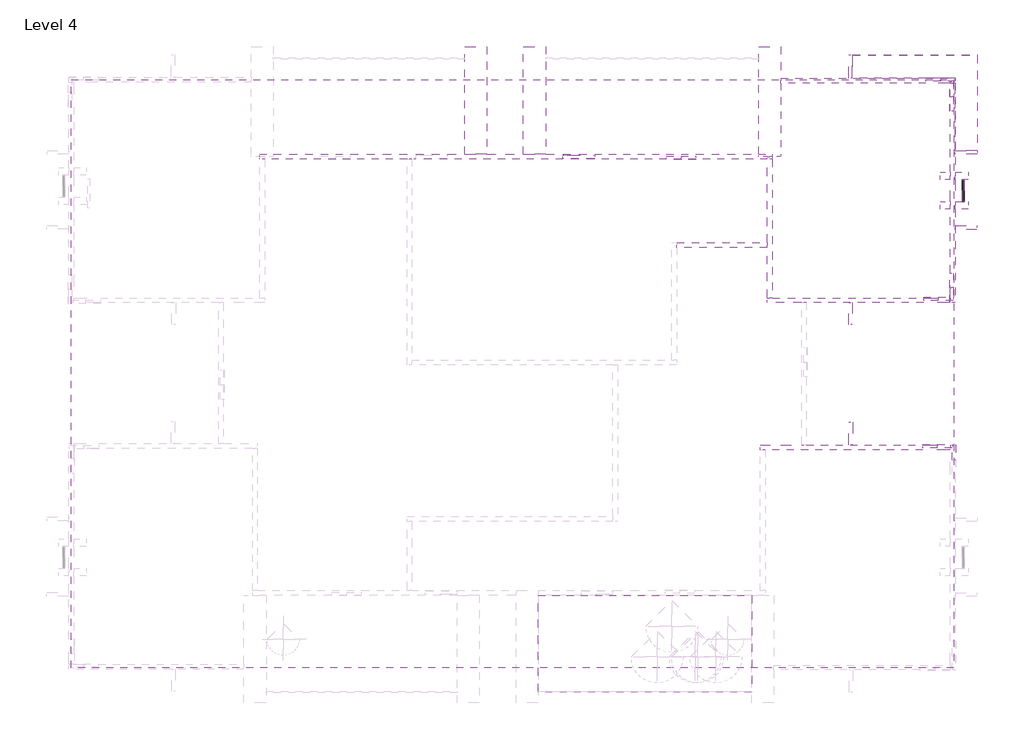
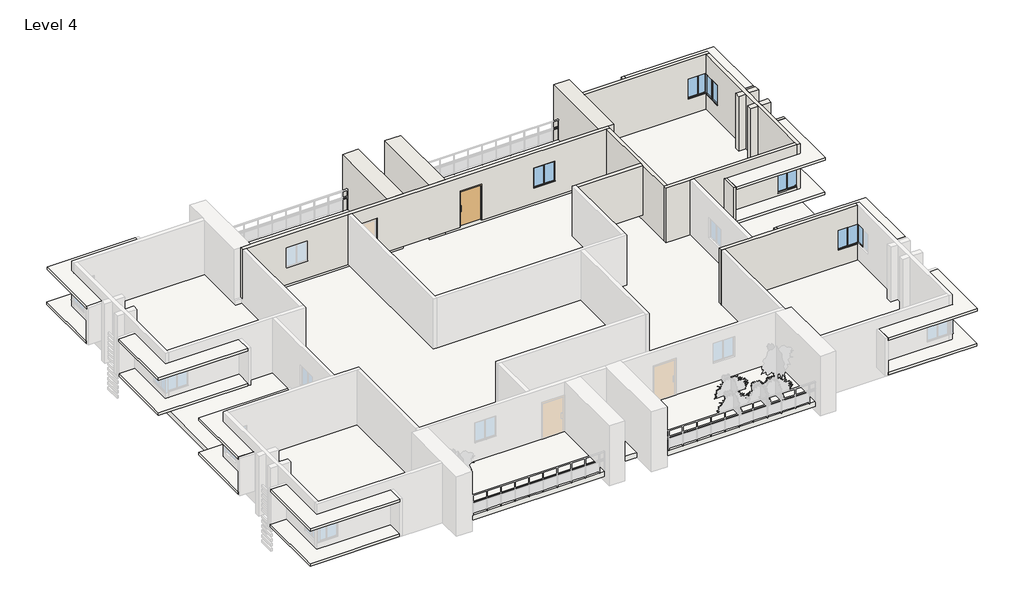
# One storey, part 3 of 4: 31 walls, 13 windows, 4 slabs, 1 door.
"""IFC4 building model written with IfcOpenShell, lengths in millimetres."""

from ifc_helpers import new_model, si_unit, frame, origin, place, context, project, spatial, polyline, outline, extrude, faceted_brep, transform, mapped, element, save
from components import door_15d3c954, window_20ff4747

model = new_model("IFC4")

# Units and contexts
model_context = context("Model", 3, world=origin())
ifc_project = project(units=[si_unit("LENGTHUNIT", "METRE", prefix="MILLI")], contexts=[model_context])

# Site, building, storey
site = spatial("IfcSite", under=ifc_project)
building = spatial("IfcBuilding", under=site)
storey = spatial("IfcBuildingStorey", under=building, Name="Level 4", Elevation=9144.0)

# Door
placement = place(None, origin())
door_shape = door_15d3c954(model_context)
element("IfcDoor", 1, ObjectType="Door-Passage-Single-Flush-Dbl_Acting : 48\" x 96\"", at=placement, inside=storey, context=model_context, shape_type="MappedRepresentation", body=[
    mapped(door_shape, transform((6249.0520665, 12804.5205944, 10972.8), x_axis=(1.0, 0.0, 0.0), y_axis=(0.0, 1.0, 0.0), z_axis=(0.0, 0.0, 1.0))),
])

# Slabs
element("IfcSlab", 2, ObjectType="Generic - 2'", at=placement, inside=storey, context=model_context, shape_type="SweptSolid", body=[
    extrude(outline(polyline([(21793.8520665, 16006.5548886), (21793.8520665, -8377.4451114), (-14782.1479335, -8377.4451114), (-14782.1479335, 16006.5548886), (21793.8520665, 16006.5548886)])), frame((0.0, 0.0, 10363.2), z_axis=(0.0, 0.0, 1.0), x_axis=(1.0, 0.0, 0.0)), (0.0, 0.0, 1.0), 304.8),
])
element("IfcSlab", 3, ObjectType="Generic - 2' gray", at=placement, inside=storey, context=model_context, shape_type="SweptSolid", body=[
    extrude(outline(polyline([(13411.8520665, -5363.830811), (13411.8520665, -9380.382663), (4572.6520665, -9380.382663), (4572.6520665, -5363.830811), (13411.8520665, -5363.830811)])), frame((0.0, 0.0, 10668.0), z_axis=(0.0, 0.0, 1.0), x_axis=(1.0, 0.0, 0.0)), (0.0, 0.0, 1.0), 304.8),
    extrude(outline(polyline([(-6704.9479335, -5363.1461695), (1219.8520665, -5363.1461695), (1219.8520665, -9380.382663), (-6704.9479335, -9380.382663), (-6704.9479335, -5363.1461695)])), frame((0.0, 0.0, 10668.0), z_axis=(0.0, 0.0, 1.0), x_axis=(1.0, 0.0, 0.0)), (0.0, 0.0, 1.0), 304.8),
    extrude(outline(polyline([(13716.6520665, 12912.4705944), (4877.4520665, 12912.4705944), (4877.4520665, 16886.1559451), (13716.6520665, 16886.1559451), (13716.6520665, 12912.4705944)])), frame((0.0, 0.0, 10668.0), z_axis=(0.0, 0.0, 1.0), x_axis=(1.0, 0.0, 0.0)), (0.0, 0.0, 1.0), 304.8),
    extrude(outline(polyline([(-6400.1479335, 12912.4705944), (-6400.1479335, 16886.1559451), (1524.6520665, 16886.1559451), (1524.6520665, 12912.4705944), (-6400.1479335, 12912.4705944)])), frame((0.0, 0.0, 10668.0), z_axis=(0.0, 0.0, 1.0), x_axis=(1.0, 0.0, 0.0)), (0.0, 0.0, 1.0), 304.8),
])
element("IfcSlab", 4, ObjectType="Generic - 6\"", at=placement, inside=storey, context=model_context, shape_type="SweptSolid", body=[
    extrude(outline(polyline([(-10616.5479335, -9354.6604699), (-15798.1479335, -9354.6604699), (-15798.1479335, -5392.2604699), (-14883.7479335, -5392.2604699), (-14883.7479335, -8338.6604699), (-14883.7479335, -8440.2604699), (-10616.5479335, -8440.2604699), (-10616.5479335, -9354.6604699)])), frame((0.0, 0.0, 11125.2), z_axis=(0.0, 0.0, 1.0), x_axis=(1.0, 0.0, 0.0)), (0.0, 0.0, 1.0), 152.4),
    extrude(outline(polyline([(-10633.1034654, 1834.0395301), (-10633.1034654, 919.6395301), (-14883.7479335, 919.6395301), (-14883.7479335, -2128.3604699), (-15775.8097154, -2128.3604699), (-15775.8097154, 1834.0395301), (-10633.1034654, 1834.0395301)])), frame((0.0, 0.0, 11125.2), z_axis=(0.0, 0.0, 1.0), x_axis=(1.0, 0.0, 0.0)), (0.0, 0.0, 1.0), 152.4),
    extrude(outline(polyline([(-10616.5479335, 5846.5548886), (-15798.1479335, 5846.5548886), (-15798.1479335, 9808.9548886), (-14883.7479335, 9808.9548886), (-14883.7479335, 6862.5548886), (-14883.7479335, 6760.9548886), (-10616.5479335, 6760.9548886), (-10616.5479335, 5846.5548886)])), frame((0.0, 0.0, 11125.2), z_axis=(0.0, 0.0, 1.0), x_axis=(1.0, 0.0, 0.0)), (0.0, 0.0, 1.0), 152.4),
    extrude(outline(polyline([(-10633.1034654, 17035.2548886), (-10633.1034654, 16120.8548886), (-14883.7479335, 16120.8548886), (-14883.7479335, 13072.8548886), (-15775.8097154, 13072.8548886), (-15775.8097154, 17035.2548886), (-10633.1034654, 17035.2548886)])), frame((0.0, 0.0, 11125.2), z_axis=(0.0, 0.0, 1.0), x_axis=(1.0, 0.0, 0.0)), (0.0, 0.0, 1.0), 152.4),
    extrude(outline(polyline([(17590.1520665, 17035.2548886), (22771.7520665, 17035.2548886), (22771.7520665, 13072.8548886), (21857.3520665, 13072.8548886), (21857.3520665, 16019.2548886), (21857.3520665, 16070.0548886), (17590.1520665, 16070.0548886), (17590.1520665, 16120.8548886), (17590.1520665, 17035.2548886)])), frame((0.0, 0.0, 11125.2), z_axis=(0.0, 0.0, 1.0), x_axis=(1.0, 0.0, 0.0)), (0.0, 0.0, 1.0), 152.4),
    extrude(outline(polyline([(17606.7075984, 5846.5548886), (17606.7075984, 6760.9548886), (21857.3520665, 6760.9548886), (21857.3520665, 9808.9548886), (22749.4138484, 9808.9548886), (22749.4138484, 5846.5548886), (17606.7075984, 5846.5548886)])), frame((0.0, 0.0, 11125.2), z_axis=(0.0, 0.0, 1.0), x_axis=(1.0, 0.0, 0.0)), (0.0, 0.0, 1.0), 152.4),
    extrude(outline(polyline([(17590.1520665, 1807.9548886), (22771.7520665, 1807.9548886), (22771.7520665, -2154.4451114), (21857.3520665, -2154.4451114), (21857.3520665, 791.9548886), (21857.3520665, 893.5548886), (17590.1520665, 893.5548886), (17590.1520665, 1807.9548886)])), frame((0.0, 0.0, 11125.2), z_axis=(0.0, 0.0, 1.0), x_axis=(1.0, 0.0, 0.0)), (0.0, 0.0, 1.0), 152.4),
    extrude(outline(polyline([(17606.7075984, -9380.7451114), (17606.7075984, -8466.3451114), (21857.3520665, -8466.3451114), (21857.3520665, -5418.3451114), (22749.4138484, -5418.3451114), (22749.4138484, -9380.7451114), (17606.7075984, -9380.7451114)])), frame((0.0, 0.0, 11125.2), z_axis=(0.0, 0.0, 1.0), x_axis=(1.0, 0.0, 0.0)), (0.0, 0.0, 1.0), 152.4),
])
element("IfcSlab", 5, ObjectType="Generic - 6\"", at=placement, inside=storey, context=model_context, shape_type="SweptSolid", body=[
    extrude(outline(polyline([(-10617.0810044, -9363.7552779), (-15798.6810044, -9363.7552779), (-15798.6810044, -5401.3552779), (-14884.2810044, -5401.3552779), (-14884.2810044, -8347.7552779), (-14884.2810044, -8449.3552779), (-10617.0810044, -8449.3552779), (-10617.0810044, -9363.7552779)])), frame((0.0, 0.0, 13258.8), z_axis=(0.0, 0.0, 1.0), x_axis=(1.0, 0.0, 0.0)), (0.0, 0.0, 1.0), 152.4),
    extrude(outline(polyline([(-10633.6365363, 1824.9447221), (-10633.6365363, 910.5447221), (-14884.2810044, 910.5447221), (-14884.2810044, -2137.4552779), (-15776.3427863, -2137.4552779), (-15776.3427863, 1824.9447221), (-10633.6365363, 1824.9447221)])), frame((0.0, 0.0, 13258.8), z_axis=(0.0, 0.0, 1.0), x_axis=(1.0, 0.0, 0.0)), (0.0, 0.0, 1.0), 152.4),
    extrude(outline(polyline([(-10617.0810044, 5837.4600805), (-15798.6810044, 5837.4600805), (-15798.6810044, 9799.8600805), (-14884.2810044, 9799.8600805), (-14884.2810044, 6853.4600805), (-14884.2810044, 6751.8600805), (-10617.0810044, 6751.8600805), (-10617.0810044, 5837.4600805)])), frame((0.0, 0.0, 13258.8), z_axis=(0.0, 0.0, 1.0), x_axis=(1.0, 0.0, 0.0)), (0.0, 0.0, 1.0), 152.4),
    extrude(outline(polyline([(-10633.6365363, 17026.1600805), (-10633.6365363, 16111.7600805), (-14884.2810044, 16111.7600805), (-14884.2810044, 13063.7600805), (-15776.3427863, 13063.7600805), (-15776.3427863, 17026.1600805), (-10633.6365363, 17026.1600805)])), frame((0.0, 0.0, 13258.8), z_axis=(0.0, 0.0, 1.0), x_axis=(1.0, 0.0, 0.0)), (0.0, 0.0, 1.0), 152.4),
    extrude(outline(polyline([(17589.6189956, 17026.1600805), (22771.2189956, 17026.1600805), (22771.2189956, 13063.7600805), (21856.8189956, 13063.7600805), (21856.8189956, 16010.1600805), (21856.8189956, 16060.9600805), (17589.6189956, 16060.9600805), (17589.6189956, 16111.7600805), (17589.6189956, 17026.1600805)])), frame((0.0, 0.0, 13258.8), z_axis=(0.0, 0.0, 1.0), x_axis=(1.0, 0.0, 0.0)), (0.0, 0.0, 1.0), 152.4),
    extrude(outline(polyline([(17606.1745274, 5837.4600805), (17606.1745274, 6751.8600805), (21856.8189956, 6751.8600805), (21856.8189956, 9799.8600805), (22748.8807774, 9799.8600805), (22748.8807774, 5837.4600805), (17606.1745274, 5837.4600805)])), frame((0.0, 0.0, 13258.8), z_axis=(0.0, 0.0, 1.0), x_axis=(1.0, 0.0, 0.0)), (0.0, 0.0, 1.0), 152.4),
    extrude(outline(polyline([(17589.6189956, 1798.8600805), (22771.2189956, 1798.8600805), (22771.2189956, -2163.5399195), (21856.8189956, -2163.5399195), (21856.8189956, 782.8600805), (21856.8189956, 884.4600805), (17589.6189956, 884.4600805), (17589.6189956, 1798.8600805)])), frame((0.0, 0.0, 13258.8), z_axis=(0.0, 0.0, 1.0), x_axis=(1.0, 0.0, 0.0)), (0.0, 0.0, 1.0), 152.4),
    extrude(outline(polyline([(17606.1745274, -9389.8399195), (17606.1745274, -8475.4399195), (21856.8189956, -8475.4399195), (21856.8189956, -5427.4399195), (22748.8807774, -5427.4399195), (22748.8807774, -9389.8399195), (17606.1745274, -9389.8399195)])), frame((0.0, 0.0, 13258.8), z_axis=(0.0, 0.0, 1.0), x_axis=(1.0, 0.0, 0.0)), (0.0, 0.0, 1.0), 152.4),
])

# Walls
element("IfcWall", 6, ObjectType="Generic - 1'", at=placement, inside=storey, context=model_context, shape_type="SweptSolid", body=[
    extrude(outline(polyline([(22386.1027846, 11871.0705944), (21857.3520665, 11871.0705944), (21857.3520665, 12175.8705944), (22386.1027846, 12175.8705944), (22386.1027846, 11871.0705944)])), frame((0.0, 0.0, 10363.2), z_axis=(0.0, 0.0, 1.0), x_axis=(1.0, 0.0, 0.0)), (0.0, 0.0, 1.0), 3657.6),
])
element("IfcWall", 7, ObjectType="Generic - 1'", at=placement, inside=storey, context=model_context, shape_type="SweptSolid", body=[
    extrude(outline(polyline([(21235.7605971, 12175.8705944), (21654.1520665, 12175.8705944), (21654.1520665, 11871.0705944), (21235.7605971, 11871.0705944), (21235.7605971, 12175.8705944)])), frame((0.0, 0.0, 10363.2), z_axis=(0.0, 0.0, 1.0), x_axis=(1.0, 0.0, 0.0)), (0.0, 0.0, 1.0), 3657.6),
])
element("IfcWall", 8, ObjectType="Generic - 1'", at=placement, inside=storey, context=model_context, shape_type="SweptSolid", body=[
    extrude(outline(polyline([(22386.1027846, 10651.8705944), (21857.3520665, 10651.8705944), (21857.3520665, 10956.6705944), (22386.1027846, 10956.6705944), (22386.1027846, 10651.8705944)])), frame((0.0, 0.0, 10363.2), z_axis=(0.0, 0.0, 1.0), x_axis=(1.0, 0.0, 0.0)), (0.0, 0.0, 1.0), 3657.6),
])
element("IfcWall", 9, ObjectType="Generic - 1'", at=placement, inside=storey, context=model_context, shape_type="SweptSolid", body=[
    extrude(outline(polyline([(21235.7605971, 10956.6705944), (21654.1520665, 10956.6705944), (21654.1520665, 10651.8705944), (21235.7605971, 10651.8705944), (21235.7605971, 10956.6705944)])), frame((0.0, 0.0, 10363.2), z_axis=(0.0, 0.0, 1.0), x_axis=(1.0, 0.0, 0.0)), (0.0, 0.0, 1.0), 3657.6),
])
element("IfcWall", 10, ObjectType="Generic - 3'", at=placement, inside=storey, context=model_context, shape_type="SweptSolid", body=[
    extrude(outline(polyline([(2439.0520665, 17382.8705944), (2439.0520665, 12912.4705944), (1524.6520665, 12912.4705944), (1524.6520665, 17382.8705944), (2439.0520665, 17382.8705944)])), frame((0.0, 0.0, 10363.2), z_axis=(0.0, 0.0, 1.0), x_axis=(1.0, 0.0, 0.0)), (0.0, 0.0, 1.0), 3657.6),
])
element("IfcWall", 11, ObjectType="Generic - 3'", at=placement, inside=storey, context=model_context, shape_type="SweptSolid", body=[
    extrude(outline(polyline([(4877.4520665, 17382.8705944), (4877.4520665, 12912.4705944), (3963.0520665, 12912.4705944), (3963.0520665, 17382.8705944), (4877.4520665, 17382.8705944)])), frame((0.0, 0.0, 10363.2), z_axis=(0.0, 0.0, 1.0), x_axis=(1.0, 0.0, 0.0)), (0.0, 0.0, 1.0), 3657.6),
])
element("IfcWall", 12, ObjectType="Generic - 3'", at=placement, inside=storey, context=model_context, shape_type="Brep", body=[
    faceted_brep([(14631.0520665, 12810.8705944, 10363.2), (14631.0520665, 15866.8548886, 10363.2), (14631.0520665, 16070.0548886, 10363.2), (14631.0520665, 17382.8705944, 10363.2), (14631.0520665, 17382.8705944, 14020.8), (14631.0520665, 16070.0548886, 14020.8), (14631.0520665, 15866.8548886, 14020.8), (14631.0520665, 12912.4705944, 14020.8), (14631.0520665, 12912.4705944, 10972.8), (14631.0520665, 12810.8705944, 10972.8), (13716.6520665, 12810.8705944, 10363.2), (13716.6520665, 12810.8705944, 10972.8), (13716.6520665, 12912.4705944, 10972.8), (13716.6520665, 12912.4705944, 14020.8), (13716.6520665, 17382.8705944, 14020.8), (13716.6520665, 17382.8705944, 10363.2), (14275.4520665, 12810.8705944, 10363.2), (14072.2520665, 12810.8705944, 10363.2), (14275.4520665, 12912.4705944, 14020.8), (14275.4520665, 12810.8705944, 10972.8), (14072.2520665, 12810.8705944, 10972.8), (14275.4520665, 12912.4705944, 10972.8)], [[[0, 1, 2, 3, 4, 5, 6, 7, 8, 9]], [[10, 11, 12, 13, 14, 15]], [[3, 2, 1, 0, 16, 17, 10, 15]], [[4, 3, 15, 14]], [[7, 6, 5, 4, 14, 13, 18]], [[0, 9, 19, 20, 11, 10, 17, 16]], [[8, 21, 12, 11, 20, 19, 9]], [[8, 7, 18, 13, 12, 21]]]),
])
element("IfcWall", 13, ObjectType="Generic - 5\"", at=placement, inside=storey, context=model_context, shape_type="SweptSolid", body=[
    extrude(outline(polyline([(22145.9857703, 10956.6705944), (22145.9857703, 11871.0705944), (22222.1857703, 11871.0705944), (22222.1857703, 10956.6705944), (22145.9857703, 10956.6705944)])), frame((0.0, 0.0, 8712.2), z_axis=(0.0, 0.0, 1.0), x_axis=(1.0, 0.0, 0.0)), (0.0, 0.0, 1.0), 152.8735856),
])
element("IfcWall", 14, ObjectType="Generic - 5\"", at=placement, inside=storey, context=model_context, shape_type="SweptSolid", body=[
    extrude(outline(polyline([(22145.9857703, 10956.6705944), (22145.9857703, 11871.0705944), (22222.1857703, 11871.0705944), (22222.1857703, 10956.6705944), (22145.9857703, 10956.6705944)])), frame((0.0, 0.0, 9017.0), z_axis=(0.0, 0.0, 1.0), x_axis=(1.0, 0.0, 0.0)), (0.0, 0.0, 1.0), 152.8735856),
])
element("IfcWall", 15, ObjectType="Generic - 5\"", at=placement, inside=storey, context=model_context, shape_type="SweptSolid", body=[
    extrude(outline(polyline([(22145.9857703, 10956.6705944), (22145.9857703, 11871.0705944), (22222.1857703, 11871.0705944), (22222.1857703, 10956.6705944), (22145.9857703, 10956.6705944)])), frame((0.0, 0.0, 9296.4), z_axis=(0.0, 0.0, 1.0), x_axis=(1.0, 0.0, 0.0)), (0.0, 0.0, 1.0), 152.8735856),
])
element("IfcWall", 16, ObjectType="Generic - 5\"", at=placement, inside=storey, context=model_context, shape_type="SweptSolid", body=[
    extrude(outline(polyline([(22145.9857703, 10956.6705944), (22145.9857703, 11871.0705944), (22222.1857703, 11871.0705944), (22222.1857703, 10956.6705944), (22145.9857703, 10956.6705944)])), frame((0.0, 0.0, 9601.2), z_axis=(0.0, 0.0, 1.0), x_axis=(1.0, 0.0, 0.0)), (0.0, 0.0, 1.0), 152.8735856),
])
element("IfcWall", 17, ObjectType="Generic - 5\"", at=placement, inside=storey, context=model_context, shape_type="SweptSolid", body=[
    extrude(outline(polyline([(22145.9857703, 10956.6705944), (22145.9857703, 11871.0705944), (22222.1857703, 11871.0705944), (22222.1857703, 10956.6705944), (22145.9857703, 10956.6705944)])), frame((0.0, 0.0, 9906.0), z_axis=(0.0, 0.0, 1.0), x_axis=(1.0, 0.0, 0.0)), (0.0, 0.0, 1.0), 152.8735856),
])
element("IfcWall", 18, ObjectType="Generic - 5\"", at=placement, inside=storey, context=model_context, shape_type="SweptSolid", body=[
    extrude(outline(polyline([(22145.9857703, 10956.6705944), (22145.9857703, 11871.0705944), (22222.1857703, 11871.0705944), (22222.1857703, 10956.6705944), (22145.9857703, 10956.6705944)])), frame((0.0, 0.0, 10210.8), z_axis=(0.0, 0.0, 1.0), x_axis=(1.0, 0.0, 0.0)), (0.0, 0.0, 1.0), 152.8735856),
])
element("IfcWall", 19, ObjectType="Generic - 5\"", at=placement, inside=storey, context=model_context, shape_type="SweptSolid", body=[
    extrude(outline(polyline([(22145.9857703, 10956.6705944), (22145.9857703, 11871.0705944), (22222.1857703, 11871.0705944), (22222.1857703, 10956.6705944), (22145.9857703, 10956.6705944)])), frame((0.0, 0.0, 10617.2), z_axis=(0.0, 0.0, 1.0), x_axis=(1.0, 0.0, 0.0)), (0.0, 0.0, 1.0), 152.8735856),
])
element("IfcWall", 20, ObjectType="Generic - 5\"", at=placement, inside=storey, context=model_context, shape_type="SweptSolid", body=[
    extrude(outline(polyline([(22145.9857703, 10956.6705944), (22145.9857703, 11871.0705944), (22222.1857703, 11871.0705944), (22222.1857703, 10956.6705944), (22145.9857703, 10956.6705944)])), frame((0.0, 0.0, 10896.6), z_axis=(0.0, 0.0, 1.0), x_axis=(1.0, 0.0, 0.0)), (0.0, 0.0, 1.0), 152.8735856),
])
element("IfcWall", 21, ObjectType="Generic - 5\"", at=placement, inside=storey, context=model_context, shape_type="SweptSolid", body=[
    extrude(outline(polyline([(22145.9857703, 10956.6705944), (22145.9857703, 11871.0705944), (22222.1857703, 11871.0705944), (22222.1857703, 10956.6705944), (22145.9857703, 10956.6705944)])), frame((0.0, 0.0, 11176.0), z_axis=(0.0, 0.0, 1.0), x_axis=(1.0, 0.0, 0.0)), (0.0, 0.0, 1.0), 152.8735856),
])
element("IfcWall", 22, ObjectType="Generic - 5\"", at=placement, inside=storey, context=model_context, shape_type="SweptSolid", body=[
    extrude(outline(polyline([(22145.9857703, 10956.6705944), (22145.9857703, 11871.0705944), (22222.1857703, 11871.0705944), (22222.1857703, 10956.6705944), (22145.9857703, 10956.6705944)])), frame((0.0, 0.0, 11480.8), z_axis=(0.0, 0.0, 1.0), x_axis=(1.0, 0.0, 0.0)), (0.0, 0.0, 1.0), 152.8735856),
])
element("IfcWall", 23, ObjectType="Generic - 5\"", at=placement, inside=storey, context=model_context, shape_type="SweptSolid", body=[
    extrude(outline(polyline([(22145.9857703, 10956.6705944), (22145.9857703, 11871.0705944), (22222.1857703, 11871.0705944), (22222.1857703, 10956.6705944), (22145.9857703, 10956.6705944)])), frame((0.0, 0.0, 11785.6), z_axis=(0.0, 0.0, 1.0), x_axis=(1.0, 0.0, 0.0)), (0.0, 0.0, 1.0), 152.8735856),
])
element("IfcWall", 24, ObjectType="Generic - 5\"", at=placement, inside=storey, context=model_context, shape_type="SweptSolid", body=[
    extrude(outline(polyline([(22145.9857703, 10956.6705944), (22145.9857703, 11871.0705944), (22222.1857703, 11871.0705944), (22222.1857703, 10956.6705944), (22145.9857703, 10956.6705944)])), frame((0.0, 0.0, 12065.0), z_axis=(0.0, 0.0, 1.0), x_axis=(1.0, 0.0, 0.0)), (0.0, 0.0, 1.0), 152.8735856),
])
element("IfcWall", 25, ObjectType="Generic - 6\"", at=placement, inside=storey, context=model_context, shape_type="SweptSolid", body=[
    extrude(outline(polyline([(22771.7520665, 12914.1048886), (21857.3520665, 12914.1048886), (21857.3520665, 13066.5048886), (22771.7520665, 13066.5048886), (22771.7520665, 12914.1048886)])), frame((0.0, 0.0, 11125.2), z_axis=(0.0, 0.0, 1.0), x_axis=(1.0, 0.0, 0.0)), (0.0, 0.0, 1.0), 2286.0),
])
element("IfcWall", 26, ObjectType="Generic - 6\"", at=placement, inside=storey, context=model_context, shape_type="SweptSolid", body=[
    extrude(outline(polyline([(17590.1520665, 17035.2548886), (17590.1520665, 16070.0548886), (17437.7520665, 16070.0548886), (17437.7520665, 17035.2548886), (17590.1520665, 17035.2548886)])), frame((0.0, 0.0, 11125.2), z_axis=(0.0, 0.0, 1.0), x_axis=(1.0, 0.0, 0.0)), (0.0, 0.0, 1.0), 2286.0),
])
element("IfcWall", 27, ObjectType="Generic - 6\"", at=placement, inside=storey, context=model_context, shape_type="SweptSolid", body=[
    extrude(outline(polyline([(22748.8807774, 9799.8600805), (21857.3520665, 9799.8600805), (21857.3520665, 9952.2600805), (22748.8807774, 9952.2600805), (22748.8807774, 9799.8600805)])), frame((0.0, 0.0, 11125.2), z_axis=(0.0, 0.0, 1.0), x_axis=(1.0, 0.0, 0.0)), (0.0, 0.0, 1.0), 2286.0),
])
element("IfcWall", 28, ObjectType="Generic - 6\"", at=placement, inside=storey, context=model_context, shape_type="SweptSolid", body=[
    extrude(outline(polyline([(17441.6075984, 5850.1600805), (17441.6075984, 6760.9548886), (17594.0075984, 6760.9548886), (17594.0075984, 5850.1600805), (17441.6075984, 5850.1600805)])), frame((0.0, 0.0, 11125.2), z_axis=(0.0, 0.0, 1.0), x_axis=(1.0, 0.0, 0.0)), (0.0, 0.0, 1.0), 2286.0),
])
element("IfcWall", 29, ObjectType="Generic - 6\"", at=placement, inside=storey, context=model_context, shape_type="SweptSolid", body=[
    extrude(outline(polyline([(17595.9689956, 1807.9548886), (17595.9689956, 868.1548886), (17443.5689956, 868.1548886), (17443.5689956, 1807.9548886), (17595.9689956, 1807.9548886)])), frame((0.0, 0.0, 11125.2), z_axis=(0.0, 0.0, 1.0), x_axis=(1.0, 0.0, 0.0)), (0.0, 0.0, 1.0), 2286.0),
])
element("IfcWall", 30, ObjectType="Generic - 8\"", at=placement, inside=storey, context=model_context, shape_type="SweptSolid", body=[
    extrude(outline(polyline([(14072.2520665, 9051.6705944), (10313.0520665, 9051.6705944), (10313.0520665, 9254.8705944), (14072.2520665, 9254.8705944), (14072.2520665, 9051.6705944)])), frame((0.0, 0.0, 10972.8), z_axis=(0.0, 0.0, 1.0), x_axis=(1.0, 0.0, 0.0)), (0.0, 0.0, 1.0), 3048.0),
])
element("IfcWall", 31, ObjectType="Generic - 8\" gray", at=placement, inside=storey, context=model_context, shape_type="Brep", body=[
    faceted_brep([(21857.3520665, 16070.0548886, 10363.2), (14631.0520665, 16070.0548886, 10363.2), (14631.0520665, 16070.0548886, 14020.8), (21857.3520665, 16070.0548886, 14020.8), (20634.9770665, 16070.0548886, 11635.4804451), (21854.1770665, 16070.0548886, 11635.4804451), (21854.1770665, 16070.0548886, 12854.6804451), (20634.9770665, 16070.0548886, 12854.6804451), (14631.0520665, 15866.8548886, 10363.2), (21654.1520665, 15866.8548886, 10363.2), (21857.3520665, 15866.8548886, 10363.2), (21857.3520665, 15866.8548886, 11617.3280277), (21857.3520665, 15866.8548886, 12836.5280277), (21857.3520665, 15866.8548886, 14020.8), (21654.1520665, 15866.8548886, 14020.8), (14631.0520665, 15866.8548886, 14020.8), (20634.9770665, 15866.8548886, 12854.6804451), (21854.1770665, 15866.8548886, 12854.6804451), (21854.1770665, 15866.8548886, 11635.4804451), (20634.9770665, 15866.8548886, 11635.4804451)], [[[0, 1, 2, 3], [4, 5, 6, 7]], [[8, 9, 10, 11, 12, 13, 14, 15], [16, 17, 18, 19]], [[1, 0, 10, 9, 8]], [[3, 2, 15, 14, 13]], [[0, 3, 13, 12, 11, 10]], [[2, 1, 8, 15]], [[18, 17, 6, 5]], [[18, 5, 4, 19]], [[16, 7, 6, 17]], [[19, 4, 7, 16]]]),
])
element("IfcWall", 32, ObjectType="Generic - 8\" gray", at=placement, inside=storey, context=model_context, shape_type="Brep", body=[
    faceted_brep([(21857.3520665, 6760.9548886, 10363.2), (21857.3520665, 10651.8705944, 10363.2), (21857.3520665, 10956.6705944, 10363.2), (21857.3520665, 11871.0705944, 10363.2), (21857.3520665, 12175.8705944, 10363.2), (21857.3520665, 15866.8548886, 10363.2), (21857.3520665, 15866.8548886, 11617.3280277), (21857.3520665, 14696.4442594, 11617.3280277), (21857.3520665, 14696.4442594, 12836.5280277), (21857.3520665, 15866.8548886, 12836.5280277), (21857.3520665, 15866.8548886, 14020.8), (21857.3520665, 12175.8705944, 14020.8), (21857.3520665, 11871.0705944, 14020.8), (21857.3520665, 10956.6705944, 14020.8), (21857.3520665, 10651.8705944, 14020.8), (21857.3520665, 6760.9548886, 14020.8), (21857.3520665, 7997.1026284, 11470.2947232), (21857.3520665, 6777.9026284, 11470.2947232), (21857.3520665, 6777.9026284, 12689.4947232), (21857.3520665, 7997.1026284, 12689.4947232), (21654.1520665, 15866.8548886, 10363.2), (21654.1520665, 12175.8705944, 10363.2), (21654.1520665, 11871.0705944, 10363.2), (21654.1520665, 10956.6705944, 10363.2), (21654.1520665, 10651.8705944, 10363.2), (21654.1520665, 6964.1548886, 10363.2), (21654.1520665, 6760.9548886, 10363.2), (21654.1520665, 6760.9548886, 11421.1450479), (21654.1520665, 6760.9548886, 12640.3450479), (21654.1520665, 6760.9548886, 14020.8), (21654.1520665, 6964.1548886, 14020.8), (21654.1520665, 10651.8705944, 14020.8), (21654.1520665, 10956.6705944, 14020.8), (21654.1520665, 11871.0705944, 14020.8), (21654.1520665, 12175.8705944, 14020.8), (21654.1520665, 15866.8548886, 14020.8), (21654.1520665, 15866.8548886, 12836.5280277), (21654.1520665, 14696.4442594, 12836.5280277), (21654.1520665, 14696.4442594, 11617.3280277), (21654.1520665, 15866.8548886, 11617.3280277), (21654.1520665, 6777.9026284, 11470.2947232), (21654.1520665, 7997.1026284, 11470.2947232), (21654.1520665, 7997.1026284, 12689.4947232), (21654.1520665, 6777.9026284, 12689.4947232)], [[[0, 1, 2, 3, 4, 5, 6, 7, 8, 9, 10, 11, 12, 13, 14, 15], [16, 17, 18, 19]], [[20, 21, 22, 23, 24, 25, 26, 27, 28, 29, 30, 31, 32, 33, 34, 35, 36, 37, 38, 39], [40, 41, 42, 43]], [[5, 4, 3, 2, 1, 0, 26, 25, 24, 23, 22, 21, 20]], [[15, 14, 13, 12, 11, 10, 35, 34, 33, 32, 31, 30, 29]], [[0, 15, 29, 28, 27, 26]], [[5, 20, 39, 6]], [[35, 10, 9, 36]], [[38, 7, 6, 39]], [[8, 7, 38, 37]], [[8, 37, 36, 9]], [[16, 41, 40, 17]], [[18, 43, 42, 19]], [[19, 42, 41, 16]], [[43, 18, 17, 40]]]),
])
element("IfcWall", 33, ObjectType="Generic - 8\" gray", at=placement, inside=storey, context=model_context, shape_type="Brep", body=[
    faceted_brep([(14072.2520665, 6760.9548886, 10363.2), (15481.9520665, 6760.9548886, 10363.2), (15685.1520665, 6760.9548886, 10363.2), (21654.1520665, 6760.9548886, 10363.2), (21654.1520665, 6760.9548886, 11421.1450479), (20541.6213445, 6760.9548886, 11421.1450479), (20541.6213445, 6760.9548886, 12640.3450479), (21654.1520665, 6760.9548886, 12640.3450479), (21654.1520665, 6760.9548886, 14020.8), (15685.1520665, 6760.9548886, 14020.8), (15481.9520665, 6760.9548886, 14020.8), (14072.2520665, 6760.9548886, 14020.8), (21654.1520665, 6964.1548886, 10363.2), (14275.4520665, 6964.1548886, 10363.2), (14072.2520665, 6964.1548886, 10363.2), (14072.2520665, 6964.1548886, 14020.8), (14275.4520665, 6964.1548886, 14020.8), (21654.1520665, 6964.1548886, 14020.8), (21654.1520665, 6964.1548886, 12640.3450479), (20541.6213445, 6964.1548886, 12640.3450479), (20541.6213445, 6964.1548886, 11421.1450479), (21654.1520665, 6964.1548886, 11421.1450479)], [[[0, 1, 2, 3, 4, 5, 6, 7, 8, 9, 10, 11]], [[12, 13, 14, 15, 16, 17, 18, 19, 20, 21]], [[3, 2, 1, 0, 14, 13, 12]], [[11, 10, 9, 8, 17, 16, 15]], [[3, 12, 21, 4]], [[17, 8, 7, 18]], [[0, 11, 15, 14]], [[4, 21, 20, 5]], [[6, 5, 20, 19]], [[6, 19, 18, 7]]]),
])
element("IfcWall", 34, ObjectType="Generic - 8\" gray", at=placement, inside=storey, context=model_context, shape_type="Brep", body=[
    faceted_brep([(13767.4520665, 664.9548886, 10363.2), (13970.6520665, 664.9548886, 10363.2), (21654.1520665, 664.9548886, 10363.2), (21654.1520665, 664.9548886, 11635.4804451), (20505.783383, 664.9548886, 11635.4804451), (20505.783383, 664.9548886, 12854.6804451), (21654.1520665, 664.9548886, 12854.6804451), (21654.1520665, 664.9548886, 14020.8), (13970.6520665, 664.9548886, 14020.8), (13767.4520665, 664.9548886, 14020.8), (21654.1520665, 868.1548886, 10363.2), (15685.1520665, 868.1548886, 10363.2), (15481.9520665, 868.1548886, 10363.2), (13767.4520665, 868.1548886, 10363.2), (13767.4520665, 868.1548886, 14020.8), (15481.9520665, 868.1548886, 14020.8), (15685.1520665, 868.1548886, 14020.8), (21654.1520665, 868.1548886, 14020.8), (21654.1520665, 868.1548886, 12854.6804451), (20505.783383, 868.1548886, 12854.6804451), (20505.783383, 868.1548886, 11635.4804451), (21654.1520665, 868.1548886, 11635.4804451), (21654.1520665, 859.364485, 11635.4804451), (21654.1520665, 859.364485, 12854.6804451)], [[[0, 1, 2, 3, 4, 5, 6, 7, 8, 9]], [[10, 11, 12, 13, 14, 15, 16, 17, 18, 19, 20, 21]], [[2, 1, 0, 13, 12, 11, 10]], [[9, 8, 7, 17, 16, 15, 14]], [[2, 10, 21, 22, 3]], [[17, 7, 6, 23, 18]], [[0, 9, 14, 13]], [[3, 22, 21, 20, 4]], [[5, 4, 20, 19]], [[5, 19, 18, 23, 6]]]),
])
element("IfcWall", 35, ObjectType="Generic - 8\" gray", at=placement, inside=storey, context=model_context, shape_type="Brep", body=[
    faceted_brep([(-6958.9479335, 12912.4705944, 14020.8), (-6400.1479335, 12912.4705944, 14020.8), (1524.6520665, 12912.4705944, 14020.8), (2439.0520665, 12912.4705944, 14020.8), (3963.0520665, 12912.4705944, 14020.8), (4877.4520665, 12912.4705944, 14020.8), (13716.6520665, 12912.4705944, 14020.8), (14275.4520665, 12912.4705944, 14020.8), (14275.4520665, 12912.4705944, 10972.8), (13716.6520665, 12912.4705944, 10972.8), (6909.4520665, 12912.4705944, 10972.8), (6909.4520665, 12912.4705944, 13208.0), (5588.6520665, 12912.4705944, 13208.0), (5588.6520665, 12912.4705944, 10972.8), (813.4520665, 12912.4705944, 10972.8), (813.4520665, 12912.4705944, 13208.0), (-507.3479335, 12912.4705944, 13208.0), (-507.3479335, 12912.4705944, 10972.8), (-6400.1479335, 12912.4705944, 10972.8), (-6958.9479335, 12912.4705944, 10972.8), (11102.1500799, 12912.4705944, 11892.0873953), (11102.1500799, 12912.4705944, 13111.2873953), (9882.9500799, 12912.4705944, 13111.2873953), (9882.9500799, 12912.4705944, 11892.0873953), (-3213.321881, 12912.4705944, 12018.2298362), (-3213.321881, 12912.4705944, 13237.4298362), (-4432.521881, 12912.4705944, 13237.4298362), (-4432.521881, 12912.4705944, 12018.2298362), (14275.4520665, 12709.2705944, 14020.8), (14072.2520665, 12709.2705944, 14020.8), (-659.7479335, 12709.2705944, 14020.8), (-862.9479335, 12709.2705944, 14020.8), (-6755.7479335, 12709.2705944, 14020.8), (-6958.9479335, 12709.2705944, 14020.8), (-6958.9479335, 12709.2705944, 10972.8), (-6755.7479335, 12709.2705944, 10972.8), (-862.9479335, 12709.2705944, 10972.8), (-659.7479335, 12709.2705944, 10972.8), (-507.3479335, 12709.2705944, 10972.8), (-507.3479335, 12709.2705944, 13208.0), (813.4520665, 12709.2705944, 13208.0), (813.4520665, 12709.2705944, 10972.8), (5588.6520665, 12709.2705944, 10972.8), (5588.6520665, 12709.2705944, 13208.0), (6909.4520665, 12709.2705944, 13208.0), (6909.4520665, 12709.2705944, 10972.8), (14072.2520665, 12709.2705944, 10972.8), (14275.4520665, 12709.2705944, 10972.8), (11102.1500799, 12709.2705944, 13111.2873953), (11102.1500799, 12709.2705944, 11892.0873953), (9882.9500799, 12709.2705944, 11892.0873953), (9882.9500799, 12709.2705944, 13111.2873953), (-3213.321881, 12709.2705944, 13237.4298362), (-3213.321881, 12709.2705944, 12018.2298362), (-4432.521881, 12709.2705944, 12018.2298362), (-4432.521881, 12709.2705944, 13237.4298362), (14275.4520665, 12810.8705944, 10972.8), (-6958.9479335, 12810.8705944, 10972.8)], [[[0, 1, 2, 3, 4, 5, 6, 7, 8, 9, 10, 11, 12, 13, 14, 15, 16, 17, 18, 19], [20, 21, 22, 23], [24, 25, 26, 27]], [[28, 29, 30, 31, 32, 33, 34, 35, 36, 37, 38, 39, 40, 41, 42, 43, 44, 45, 46, 47], [48, 49, 50, 51], [52, 53, 54, 55]], [[8, 56, 47, 46, 45, 10, 9]], [[34, 57, 19, 18, 17, 38, 37, 36, 35]], [[13, 42, 41, 14]], [[7, 6, 5, 4, 3, 2, 1, 0, 33, 32, 31, 30, 29, 28]], [[8, 7, 28, 47, 56]], [[0, 19, 57, 34, 33]], [[49, 20, 23, 50]], [[21, 20, 49, 48]], [[21, 48, 51, 22]], [[22, 51, 50, 23]], [[53, 24, 27, 54]], [[25, 24, 53, 52]], [[25, 52, 55, 26]], [[26, 55, 54, 27]], [[44, 11, 10, 45]], [[11, 44, 43, 12]], [[12, 43, 42, 13]], [[40, 15, 14, 41]], [[15, 40, 39, 16]], [[16, 39, 38, 17]]]),
])
element("IfcWall", 36, ObjectType="Generic - 8\" gray", at=placement, inside=storey, context=model_context, shape_type="Brep", body=[
    faceted_brep([(14275.4520665, 6964.1548886, 10363.2), (14275.4520665, 12810.8705944, 10363.2), (14275.4520665, 12810.8705944, 10972.8), (14275.4520665, 12709.2705944, 10972.8), (14275.4520665, 12709.2705944, 14020.8), (14275.4520665, 6964.1548886, 14020.8), (14072.2520665, 6964.1548886, 10363.2), (14072.2520665, 6964.1548886, 14020.8), (14072.2520665, 9051.6705944, 14020.8), (14072.2520665, 9254.8705944, 14020.8), (14072.2520665, 12709.2705944, 14020.8), (14072.2520665, 12709.2705944, 10972.8), (14072.2520665, 12810.8705944, 10972.8), (14072.2520665, 12810.8705944, 10363.2)], [[[0, 1, 2, 3, 4, 5]], [[6, 7, 8, 9, 10, 11, 12, 13]], [[1, 0, 6, 13]], [[5, 4, 10, 9, 8, 7]], [[0, 5, 7, 6]], [[2, 1, 13, 12]], [[11, 3, 2, 12]], [[4, 3, 11, 10]]]),
])

# Windows
window_shape = window_20ff4747(model_context)
element("IfcWindow", 37, ObjectType="Instance - Fixed : 24\" x 48\"", at=placement, inside=storey, context=model_context, shape_type="MappedRepresentation", body=[
    mapped(window_shape, transform((21587.4770665, 15968.4548886, 10721.0804451), x_axis=(1.0, 0.0, 0.0), y_axis=(0.0, 1.0, 0.0), z_axis=(0.0, 0.0, 1.0))),
])
element("IfcWindow", 38, ObjectType="Instance - Fixed : 24\" x 48\"", at=placement, inside=storey, context=model_context, shape_type="MappedRepresentation", body=[
    mapped(window_shape, transform((20977.8770665, 15968.4548886, 10721.0804451), x_axis=(1.0, 0.0, 0.0), y_axis=(0.0, 1.0, 0.0), z_axis=(0.0, 0.0, 1.0))),
])
element("IfcWindow", 39, ObjectType="Instance - Fixed : 24\" x 48\"", at=placement, inside=storey, context=model_context, shape_type="MappedRepresentation", body=[
    mapped(window_shape, transform((21755.7520665, 15648.9442594, 10702.9280277), x_axis=(0.0, 1.0, 0.0), y_axis=(-1.0, 0.0, 0.0), z_axis=(0.0, 0.0, 1.0))),
])
element("IfcWindow", 40, ObjectType="Instance - Fixed : 24\" x 48\"", at=placement, inside=storey, context=model_context, shape_type="MappedRepresentation", body=[
    mapped(window_shape, transform((21755.7520665, 15039.3442594, 10702.9280277), x_axis=(0.0, 1.0, 0.0), y_axis=(-1.0, 0.0, 0.0), z_axis=(0.0, 0.0, 1.0))),
])
element("IfcWindow", 41, ObjectType="Instance - Fixed : 24\" x 48\"", at=placement, inside=storey, context=model_context, shape_type="MappedRepresentation", body=[
    mapped(window_shape, transform((21458.283383, 766.5548886, 10721.0804451), x_axis=(1.0, 0.0, 0.0), y_axis=(0.0, 1.0, 0.0), z_axis=(0.0, 0.0, 1.0))),
])
element("IfcWindow", 42, ObjectType="Instance - Fixed : 24\" x 48\"", at=placement, inside=storey, context=model_context, shape_type="MappedRepresentation", body=[
    mapped(window_shape, transform((20848.683383, 766.5548886, 10721.0804451), x_axis=(1.0, 0.0, 0.0), y_axis=(0.0, 1.0, 0.0), z_axis=(0.0, 0.0, 1.0))),
])
element("IfcWindow", 43, ObjectType="Instance - Fixed : 24\" x 48\"", at=placement, inside=storey, context=model_context, shape_type="MappedRepresentation", body=[
    mapped(window_shape, transform((21755.7520665, 516.464485, 10721.0804451), x_axis=(0.0, -1.0, 0.0), y_axis=(1.0, 0.0, 0.0), z_axis=(0.0, 0.0, 1.0))),
])
element("IfcWindow", 44, ObjectType="Instance - Fixed : 24\" x 48\"", at=placement, inside=storey, context=model_context, shape_type="MappedRepresentation", body=[
    mapped(window_shape, transform((21755.7520665, 7730.4026284, 10555.8947232), x_axis=(0.0, 1.0, 0.0), y_axis=(-1.0, 0.0, 0.0), z_axis=(0.0, 0.0, 1.0))),
])
element("IfcWindow", 45, ObjectType="Instance - Fixed : 24\" x 48\"", at=placement, inside=storey, context=model_context, shape_type="MappedRepresentation", body=[
    mapped(window_shape, transform((21755.7520665, 7120.8026284, 10555.8947232), x_axis=(0.0, 1.0, 0.0), y_axis=(-1.0, 0.0, 0.0), z_axis=(0.0, 0.0, 1.0))),
])
element("IfcWindow", 46, ObjectType="Instance - Fixed : 24\" x 48\"", at=placement, inside=storey, context=model_context, shape_type="MappedRepresentation", body=[
    mapped(window_shape, transform((21494.1213445, 6862.5548886, 10506.7450479), x_axis=(1.0, 0.0, 0.0), y_axis=(0.0, 1.0, 0.0), z_axis=(0.0, 0.0, 1.0))),
])
element("IfcWindow", 47, ObjectType="Instance - Fixed : 24\" x 48\"", at=placement, inside=storey, context=model_context, shape_type="MappedRepresentation", body=[
    mapped(window_shape, transform((20884.5213445, 6862.5548886, 10506.7450479), x_axis=(1.0, 0.0, 0.0), y_axis=(0.0, 1.0, 0.0), z_axis=(0.0, 0.0, 1.0))),
])
element("IfcWindow", 48, ObjectType="Instance - Fixed : 24\" x 48\"", at=placement, inside=storey, context=model_context, shape_type="MappedRepresentation", body=[
    mapped(window_shape, transform((10149.6500799, 12810.8705944, 10977.6873953), x_axis=(-1.0, 0.0, 0.0), y_axis=(0.0, -1.0, 0.0), z_axis=(0.0, 0.0, 1.0))),
])
element("IfcWindow", 49, ObjectType="Instance - Fixed : 24\" x 48\"", at=placement, inside=storey, context=model_context, shape_type="MappedRepresentation", body=[
    mapped(window_shape, transform((10759.2500799, 12810.8705944, 10977.6873953), x_axis=(-1.0, 0.0, 0.0), y_axis=(0.0, -1.0, 0.0), z_axis=(0.0, 0.0, 1.0))),
])

save(model, "model.ifc")

# Revit data of these elements
# Type "Door-Passage-Single-Flush-Dbl_Acting : 48\" x 96\""
#   Type Mark = "12"
#   Assembly Code = "B2030200"
#   Analytic Construction = "Wooden"
#   Thickness = 0' - 1 3/4"
#   Thermal Resistance (R) = 2.5876 (h·ft²·°F)/BTU
#   Swing Angle [instance default] = 45.00°
#   Strike Height = 3' - 4"
#   Rough Width [instance default] = 4' - 4"
#   Rough Height [instance default] = 7' - 4"
#   MF Opening Height [instance default] = 0' - 4"
#   MF Opening Width [instance default] = 0' - 4"
#   Inset Calculate [instance default] = 0' - 4"
#   Masonry Inset [instance default] = 0' - 1"
#   Height = 7' - 0"
#   Width = 4' - 0"
#   Heat Transfer Coefficient (U) = 0.3865 BTU/(h·ft²·°F)
#   Masonry Frame Depth = 0' - 5 3/4"
#   Masonry Frame [instance default] = yes
#   Function = 1
#   Dry Wall Frame [instance default] = no
#   Panel Material = Wood - Birch
#   Frame Material = Metal - Paint Finish - Grey
#   Door Handle Material = Aluminum
#   Visual Light Transmittance = 0
#   Solar Heat Gain Coefficient = 0
#   Wall Closure = (empty or 0)
# Type "Generic - 2'"
#   Assembly Code = "B1010"
#   Function = 0
#   Layers, outside or top first: 1' - 0" "Metal - Painted - Grey" (function 1)
# Type "Generic - 2' gray"
#   Assembly Code = "B1010"
#   Function = 0
#   Layers, outside or top first: 1' - 0" "Rigid insulation" (function 1)
# Type "Generic - 6\""
#   Assembly Code = "B1010"
#   Function = 0
#   Layers, outside or top first: 0' - 6" "Metal - Painted - Grey" (function 1)
# Type "Generic - 1'"
#   Assembly Code = "B2010"
#   Layers, outside or top first: 1' - 0" "Metal - Painted - Grey" (function 1)
# Type "Generic - 3'"
#   Assembly Code = "B2010"
#   Layers, outside or top first: 3' - 0" "Metal - Painted - Grey" (function 1)
# Type "Generic - 5\""
#   Assembly Code = "B2010"
#   Layers, outside or top first: 0' - 3" "Oak Flooring" (function 1)
# Type "Generic - 6\""
#   Assembly Code = "B2010"
#   Layers, outside or top first: 0' - 6" "Metal - Painted - Grey" (function 1)
# Type "Generic - 8\""
#   Assembly Code = "B2010"
#   Layers, outside or top first: 0' - 8" no material (function 1)
# Type "Generic - 8\" gray"
#   Assembly Code = "B2010"
#   Layers, outside or top first: 0' - 8" "Parking Stripe" (function 1)
# Type "Instance - Fixed : 24\" x 48\""
#   Type Mark = "11"
#   Construction Type Id = "GSP4R"
#   Assembly Code = "B2020100"
#   Analytic Construction = "1/8 in Pilkington single glazing"
#   Visual Light Transmittance = 0.9
#   Thermal Resistance (R) = 0.8466 (h·ft²·°F)/BTU
#   Solar Heat Gain Coefficient = 0.86
#   Heat Transfer Coefficient (U) = 1.1812 BTU/(h·ft²·°F)
#   Height [instance default] = 4' - 0"
#   Default Sill Height = 3' - 0"
#   Width [instance default] = 2' - 0"
#   Window Inset = 0' - 2"
#   Define Thermal Properties by = 1
#   Glass Pane Material = Glass
#   Sash Material = Iron, Ductile
#   Wall Closure = (empty or 0)
# Element 1 (IfcDoor, "Door-Passage-Single-Flush-Dbl_Acting : 48\" x 96\"")
#   Swing Angle = 45.00°
#   Rough Width = 4' - 4"
#   Rough Height = 7' - 4"
#   Masonry Inset = 0' - 1"
#   MF Opening Width = 0' - 4"
#   MF Opening Height = 0' - 4"
#   Inset Calculate = 0' - 4"
#   Masonry Frame = yes
#   Dry Wall Frame = no
#   Phase Created = New Construction
#   Materials on its faces: "Aluminum", "Metal - Paint Finish - Grey", "Wood - Birch"
# Element 2 (IfcSlab, "Generic - 2'")
#   Height Offset From Level = 5' - 0"
#   Phase Created = New Construction
#   Materials on its faces: "Metal - Painted - Grey"
# Element 3 (IfcSlab, "Generic - 2' gray")
#   Height Offset From Level = 6' - 0"
#   Phase Created = New Construction
#   Materials on its faces: "Rigid insulation"
# Element 4 (IfcSlab, "Generic - 6\"")
#   built-in parameter 1001955 = -1.5708 (stored number, unit not read)
#   Height Offset From Level = 7' - 0"
#   Phase Created = New Construction
#   Materials on its faces: "Metal - Painted - Grey"
# Element 5 (IfcSlab, "Generic - 6\"")
#   built-in parameter 1001955 = -1.5708 (stored number, unit not read)
#   Height Offset From Level = 14' - 0"
#   Phase Created = New Construction
#   Materials on its faces: "Metal - Painted - Grey"
# Elements 6, 7, 8, 9 (IfcWall, "Generic - 1'")
#   built-in parameter 1001111 = 4' - 0"
#   Top Offset = 0' - 0"
#   Base Offset = 4' - 0"
#   Unconnected Height = 12' - 0"
#   wall height = 12' - 0"
#   Phase Created = New Construction
#   Base Constraint = Level 4
#   Materials on its faces: "Metal - Painted - Grey"
# Elements 10, 11, 12 (IfcWall, "Generic - 3'")
#   built-in parameter 1001111 = 4' - 0"
#   Top Offset = 0' - 0"
#   Base Offset = 4' - 0"
#   Unconnected Height = 12' - 0"
#   wall height = 12' - 0"
#   Phase Created = New Construction
#   Base Constraint = Level 4
#   Materials on its faces: "Metal - Painted - Grey", "EIFS, Exterior Insulation"
# Element 13 (IfcWall, "Generic - 5\"")
#   built-in parameter 1001111 = -1' - 5"
#   Top Offset = -10' - 10.98135"
#   Base Offset = -1' - 5"
#   wall height = 0' - 6.01865"
#   Phase Created = New Construction
#   Base Constraint = Level 4
#   Top Constraint = Level 5
#   Materials on its faces: "Oak Flooring"
# Element 14 (IfcWall, "Generic - 5\"")
#   built-in parameter 1001111 = -0' - 5"
#   Top Offset = -9' - 10.98135"
#   Base Offset = -0' - 5"
#   wall height = 0' - 6.01865"
#   Phase Created = New Construction
#   Base Constraint = Level 4
#   Top Constraint = Level 5
#   Materials on its faces: "Oak Flooring"
# Element 15 (IfcWall, "Generic - 5\"")
#   built-in parameter 1001111 = 0' - 6"
#   Top Offset = -8' - 11.98135"
#   Base Offset = 0' - 6"
#   wall height = 0' - 6.01865"
#   Phase Created = New Construction
#   Base Constraint = Level 4
#   Top Constraint = Level 5
#   Materials on its faces: "Oak Flooring"
# Element 16 (IfcWall, "Generic - 5\"")
#   built-in parameter 1001111 = 1' - 6"
#   Top Offset = -7' - 11.98135"
#   Base Offset = 1' - 6"
#   wall height = 0' - 6.01865"
#   Phase Created = New Construction
#   Base Constraint = Level 4
#   Top Constraint = Level 5
#   Materials on its faces: "Oak Flooring"
# Element 17 (IfcWall, "Generic - 5\"")
#   built-in parameter 1001111 = 2' - 6"
#   Top Offset = -6' - 11.98135"
#   Base Offset = 2' - 6"
#   wall height = 0' - 6.01865"
#   Phase Created = New Construction
#   Base Constraint = Level 4
#   Top Constraint = Level 5
#   Materials on its faces: "Oak Flooring"
# Element 18 (IfcWall, "Generic - 5\"")
#   built-in parameter 1001111 = 3' - 6"
#   Top Offset = -5' - 11.98135"
#   Base Offset = 3' - 6"
#   wall height = 0' - 6.01865"
#   Phase Created = New Construction
#   Base Constraint = Level 4
#   Top Constraint = Level 5
#   Materials on its faces: "Oak Flooring"
# Element 19 (IfcWall, "Generic - 5\"")
#   built-in parameter 1001111 = 4' - 10"
#   Top Offset = -4' - 7.98135"
#   Base Offset = 4' - 10"
#   wall height = 0' - 6.01865"
#   Phase Created = New Construction
#   Base Constraint = Level 4
#   Top Constraint = Level 5
#   Materials on its faces: "Oak Flooring"
# Element 20 (IfcWall, "Generic - 5\"")
#   built-in parameter 1001111 = 5' - 9"
#   Top Offset = -3' - 8.98135"
#   Base Offset = 5' - 9"
#   wall height = 0' - 6.01865"
#   Phase Created = New Construction
#   Base Constraint = Level 4
#   Top Constraint = Level 5
#   Materials on its faces: "Oak Flooring"
# Element 21 (IfcWall, "Generic - 5\"")
#   built-in parameter 1001111 = 6' - 8"
#   Top Offset = -2' - 9.98135"
#   Base Offset = 6' - 8"
#   wall height = 0' - 6.01865"
#   Phase Created = New Construction
#   Base Constraint = Level 4
#   Top Constraint = Level 5
#   Materials on its faces: "Oak Flooring"
# Element 22 (IfcWall, "Generic - 5\"")
#   built-in parameter 1001111 = 7' - 8"
#   Top Offset = -1' - 9.98135"
#   Base Offset = 7' - 8"
#   wall height = 0' - 6.01865"
#   Phase Created = New Construction
#   Base Constraint = Level 4
#   Top Constraint = Level 5
#   Materials on its faces: "Oak Flooring"
# Element 23 (IfcWall, "Generic - 5\"")
#   built-in parameter 1001111 = 8' - 8"
#   Top Offset = -0' - 9.98135"
#   Base Offset = 8' - 8"
#   wall height = 0' - 6.01865"
#   Phase Created = New Construction
#   Base Constraint = Level 4
#   Top Constraint = Level 5
#   Materials on its faces: "Oak Flooring"
# Element 24 (IfcWall, "Generic - 5\"")
#   built-in parameter 1001111 = 9' - 7"
#   Top Offset = 0' - 1.01865"
#   Base Offset = 9' - 7"
#   wall height = 0' - 6.01865"
#   Phase Created = New Construction
#   Base Constraint = Level 4
#   Top Constraint = Level 5
#   Materials on its faces: "Oak Flooring"
# Elements 25, 26, 27, 28, 29 (IfcWall, "Generic - 6\"")
#   built-in parameter 1001111 = 6' - 6"
#   Top Offset = 0' - 0"
#   Base Offset = 6' - 6"
#   Unconnected Height = 7' - 6"
#   wall height = 7' - 6"
#   Phase Created = New Construction
#   Base Constraint = Level 4
#   Materials on its faces: "Metal - Painted - Grey"
# Element 30 (IfcWall, "Generic - 8\"")
#   built-in parameter 1001111 = 6' - 0"
#   Top Offset = 0' - 0"
#   Base Offset = 6' - 0"
#   Unconnected Height = 10' - 0"
#   wall height = 10' - 0"
#   Phase Created = New Construction
#   Base Constraint = Level 4
#   Materials on its faces: "Default Wall"
# Elements 31, 32, 33, 34, 36 (IfcWall, "Generic - 8\" gray")
#   built-in parameter 1001111 = 4' - 0"
#   Top Offset = 0' - 0"
#   Base Offset = 4' - 0"
#   Unconnected Height = 12' - 0"
#   wall height = 12' - 0"
#   Phase Created = New Construction
#   Base Constraint = Level 4
#   Materials on its faces: "Parking Stripe"
# Element 35 (IfcWall, "Generic - 8\" gray")
#   built-in parameter 1001111 = 6' - 0"
#   Top Offset = 0' - 0"
#   Base Offset = 6' - 0"
#   Unconnected Height = 10' - 0"
#   wall height = 10' - 0"
#   Phase Created = New Construction
#   Base Constraint = Level 4
#   Materials on its faces: "Parking Stripe"
# Element 37 (IfcWindow, "Instance - Fixed : 24\" x 48\"")
#   Mark = "91"
#   Width = 2' - 0"
#   Height = 4' - 0"
#   Phase Created = New Construction
#   Materials on its faces: "Iron, Ductile", "Glass"
# Element 38 (IfcWindow, "Instance - Fixed : 24\" x 48\"")
#   Mark = "92"
#   Width = 2' - 0"
#   Height = 4' - 0"
#   Phase Created = New Construction
#   Materials on its faces: "Iron, Ductile", "Glass"
# Element 39 (IfcWindow, "Instance - Fixed : 24\" x 48\"")
#   Mark = "93"
#   Width = 2' - 0"
#   Height = 4' - 0"
#   Phase Created = New Construction
#   Materials on its faces: "Iron, Ductile", "Glass"
# Element 40 (IfcWindow, "Instance - Fixed : 24\" x 48\"")
#   Mark = "94"
#   Width = 2' - 0"
#   Height = 4' - 0"
#   Phase Created = New Construction
#   Materials on its faces: "Iron, Ductile", "Glass"
# Element 41 (IfcWindow, "Instance - Fixed : 24\" x 48\"")
#   Mark = "95"
#   Width = 2' - 0"
#   Height = 4' - 0"
#   Phase Created = New Construction
#   Materials on its faces: "Iron, Ductile", "Glass"
# Element 42 (IfcWindow, "Instance - Fixed : 24\" x 48\"")
#   Mark = "96"
#   Width = 2' - 0"
#   Height = 4' - 0"
#   Phase Created = New Construction
#   Materials on its faces: "Iron, Ductile", "Glass"
# Element 43 (IfcWindow, "Instance - Fixed : 24\" x 48\"")
#   Mark = "98"
#   Width = 2' - 0"
#   Height = 4' - 0"
#   Phase Created = New Construction
#   Materials on its faces: "Iron, Ductile", "Glass"
# Element 44 (IfcWindow, "Instance - Fixed : 24\" x 48\"")
#   Mark = "119"
#   Width = 2' - 0"
#   Height = 4' - 0"
#   Phase Created = New Construction
#   Materials on its faces: "Iron, Ductile", "Glass"
# Element 45 (IfcWindow, "Instance - Fixed : 24\" x 48\"")
#   Mark = "120"
#   Width = 2' - 0"
#   Height = 4' - 0"
#   Phase Created = New Construction
#   Materials on its faces: "Iron, Ductile", "Glass"
# Element 46 (IfcWindow, "Instance - Fixed : 24\" x 48\"")
#   Mark = "121"
#   Width = 2' - 0"
#   Height = 4' - 0"
#   Phase Created = New Construction
#   Materials on its faces: "Iron, Ductile", "Glass"
# Element 47 (IfcWindow, "Instance - Fixed : 24\" x 48\"")
#   Mark = "122"
#   Width = 2' - 0"
#   Height = 4' - 0"
#   Phase Created = New Construction
#   Materials on its faces: "Iron, Ductile", "Glass"
# Element 48 (IfcWindow, "Instance - Fixed : 24\" x 48\"")
#   Mark = "123"
#   Width = 2' - 0"
#   Height = 4' - 0"
#   Phase Created = New Construction
#   Materials on its faces: "Iron, Ductile", "Glass"
# Element 49 (IfcWindow, "Instance - Fixed : 24\" x 48\"")
#   Mark = "124"
#   Width = 2' - 0"
#   Height = 4' - 0"
#   Phase Created = New Construction
#   Materials on its faces: "Iron, Ductile", "Glass"
# Materials
#   "Wood - Birch": class "Wood", colour RGB 166 116 52, transparency 0, Cost = 0
#   "Metal - Paint Finish - Grey": class "Paint", colour RGB 104 104 104, transparency 0, Cost = 0
#   "Aluminum": class "Metal", colour RGB 247 247 247, transparency 0, Description = "Aluminum 6061", Cost = 0
#   "Metal - Painted - Grey": class "Paint", colour RGB 104 104 104, transparency 0, Cost = 0
#   "Rigid insulation": class "Generic", colour RGB 127 127 127, transparency 0, Description = "Rigid foam insulation board", Cost = 0
#   "Oak Flooring": class "Wood", colour RGB 216 169 114, transparency 0, Description = "Quercus Rubra", Cost = 0
#   "Parking Stripe": class "Paint", colour RGB 250 250 91, transparency 0, Cost = 0
#   "Glass": class "Glass", colour RGB 0 128 192, transparency 0.75, Description = "Soda Lime Glass", Cost = 0
#   "Iron, Ductile": class "Metal", colour RGB 0 0 0, transparency 0, Description = "Ductile cast iron", Cost = 0
#   "EIFS, Exterior Insulation": class "Generic", colour RGB 127 127 127, transparency 0, Description = "EIFS - Exterior Insulation", Cost = 0
#   "Default Wall": colour RGB 128 128 128, transparency 0
